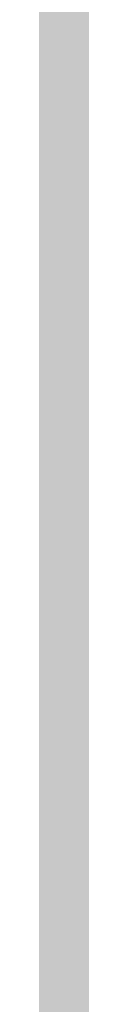
# Model space of a CAD drawing. Units: inches. Extents: x 2083 to 3317, y 1141 to 2115.
# Tile 180 of 256: x 3126.95594 to 3126.95825, y 1263.29018 to 1263.35483. Entities that reach past the tile are written whole.
import ezdxf

# ---------------------------------------------------------------- set-up
doc = ezdxf.new("R2010")
doc.units = ezdxf.units.IN
doc.layers.add('A-ANNO-DIMS', color=2, linetype='Continuous', lineweight=18)
doc.layers.add('A-WALL-PATT', color=251, linetype='Continuous', lineweight=13, true_color=0x636466)
doc.styles.get("Standard").update_dxf_attribs({"font": 'arial.ttf'})
doc.dimstyles.new('ISO-25', dxfattribs={"dimtxt": 12, "dimasz": 12, "dimexe": 1.25, "dimexo": 0.625, "dimtad": 1, "dimlunit": 3, "dimtxsty": 'Standard', "dimcen": 2.5, "dimadec": 0, "dimazin": 0, "dimtfac": 1, "dimtmove": 0, "dimatfit": 3, "dimfxl": 1, "dimarcsym": 0})

# ---------------------------------------------------------------- blocks, each defined once
blk = doc.blocks.new('*D26')
at = {"layer": 'A-ANNO-DIMS', "color": 0, "lineweight": -2, "transparency": 16777216}
for p, q in [((3088.985844, 1274.915092), (3088.985844, 1270.951963)), ((3111.240037, 1274.915092), (3111.240037, 1270.951963)), ((3076.985844, 1272.201963), (2840.262447, 1272.201963)), ((3111.240037, 1272.201963), (3088.985844, 1272.201963)), ((3123.240037, 1272.201963), (3135.240037, 1272.201963))]:
    blk.add_line(p, q, dxfattribs=at)
at = {"layer": 'A-ANNO-DIMS', "color": 0, "transparency": 16777216}
for points in [[(3076.985844, 1274.201963), (3076.985844, 1270.201963), (3088.985844, 1272.201963)], [(3123.240037, 1274.201963), (3123.240037, 1270.201963), (3111.240037, 1272.201963)]]:
    blk.add_solid(points, dxfattribs=at)
at = {"layer": 'Defpoints', "color": 0, "transparency": 16777216}
for p in [(3088.985844, 1275.540092), (3111.240037, 1275.540092), (3088.985844, 1272.201963)]:
    blk.add_point(p, dxfattribs=at)
at = {"layer": 'A-ANNO-DIMS', "color": 0, "transparency": 16777216, "insert": (2952.624146, 1279.031602), "char_height": 12, "attachment_point": 5}
blk.add_mtext('NIGHTSTAND 1\'-10 1/2" TYP.', dxfattribs=at)
blk = doc.blocks.new('*D27')
at = {"layer": 'A-ANNO-DIMS', "color": 0, "lineweight": -2, "transparency": 16777216}
for p, q in [((3114.578165, 1309.794285), (3114.578165, 1321.794285)), ((3111.865037, 1297.794285), (3115.828165, 1297.794285)), ((3114.578165, 1297.794285), (3114.578165, 1275.540092)), ((3111.865037, 1275.540092), (3115.828165, 1275.540092)), ((3114.578165, 1263.540092), (3114.578165, 1140.988591))]:
    blk.add_line(p, q, dxfattribs=at)
at = {"layer": 'A-ANNO-DIMS', "color": 0, "transparency": 16777216}
for points in [[(3112.578165, 1309.794285), (3116.578165, 1309.794285), (3114.578165, 1297.794285)], [(3112.578165, 1263.540092), (3116.578165, 1263.540092), (3114.578165, 1275.540092)]]:
    blk.add_solid(points, dxfattribs=at)
at = {"layer": 'Defpoints', "color": 0, "transparency": 16777216}
for p in [(3111.240037, 1297.794285), (3111.240037, 1275.540092), (3114.578165, 1275.540092)]:
    blk.add_point(p, dxfattribs=at)
at = {"layer": 'A-ANNO-DIMS', "color": 0, "transparency": 16777216, "insert": (3107.748527, 1196.264342), "char_height": 12, "attachment_point": 5, "rotation": 90}
blk.add_mtext('1\'-10 1/2" TYP.', dxfattribs=at)

msp = doc.modelspace()

# ---------------------------------------------------------------- hatches: boundary and pattern name
at = {"layer": 'A-WALL-PATT'}
h = msp.add_hatch(color=256, dxfattribs=at)
h.dxf.hatch_style = 1
h.paths.add_polyline_path([(3126.959783, 2020.76136), (2748.959783, 2020.76136), (2604.959783, 2020.76136), (2226.959783, 2020.76136), (2226.959783, 1702.76136), (2466.959783, 1702.76136), (2466.959783, 1582.76136), (2418.959783, 1582.76136), (2418.959783, 1477.76136), (2226.959783, 1477.76136), (2226.959783, 1263.26136), (2544.959783, 1263.26136), (2544.959783, 1411.76136), (2604.959783, 1411.76136), (2685.959783, 1411.76136), (2685.959783, 1420.76136), (2604.959783, 1420.76136), (2604.959783, 1573.76136), (2604.959783, 1702.76136), (2604.959783, 2011.76136), (2748.959783, 2011.76136), (2748.959783, 1702.76136), (2862.959783, 1702.76136), (2862.959783, 1621.76136), (2871.959783, 1621.76136), (2871.959783, 1702.76136), (2883.959783, 1702.76136), (2883.959783, 1706.939459, -0.026459), (2883.959783, 1711.76136), (2757.959783, 1711.76136), (2757.959783, 1807.76136), (2787.959783, 1807.76136), (2787.959783, 1812.26136), (2757.959783, 1812.26136), (2757.959783, 2011.76136), (2877.959783, 2011.76136), (2877.959783, 1812.26136), (2847.959783, 1812.26136), (2847.959783, 1807.76136), (2889.835742, 1807.76136), (2889.835742, 1812.26136), (2882.459783, 1812.26136), (2882.459783, 2011.76136), (3117.959783, 2011.76136), (3117.959783, 1812.26136), (2937.835742, 1812.26136), (2937.835742, 1807.76136), (2995.709783, 1807.76136), (2995.709783, 1796.117666), (3000.209783, 1796.117666), (3000.209783, 1807.76136), (3117.959783, 1807.76136), (3117.959783, 1711.76136), (3000.209783, 1711.76136), (3000.209783, 1760.117666), (2998.572705, 1760.117666, -0.020711), (2995.709783, 1760.117666), (2995.709783, 1711.76136), (2931.959783, 1711.76136), (2931.959783, 1702.76136), (3126.959783, 1702.76136)])
h.paths.add_polyline_path([(2471.459783, 2011.76136), (2471.459783, 1810.01136), (2462.716936, 1810.01136), (2462.716936, 1805.51136), (2505.959783, 1805.51136), (2505.959783, 1810.01136), (2475.959783, 1810.01136), (2475.959783, 2011.76136), (2595.959783, 2011.76136), (2595.959783, 1810.01136), (2565.959783, 1810.01136), (2565.959783, 1805.51136), (2595.959783, 1805.51136), (2595.959783, 1711.76136), (2235.959783, 1711.76136), (2235.959783, 1805.51136), (2353.709783, 1805.51136), (2353.709783, 1796.054162), (2358.209783, 1796.054162), (2358.209783, 1805.51136), (2414.716936, 1805.51136), (2414.716936, 1810.01136), (2235.959783, 1810.01136), (2235.959783, 2011.76136)], flags=16)
h.paths.add_polyline_path([(2270.204734, 1994.610008), (2270.204734, 1970.610008), (2246.204734, 1970.610008), (2246.204734, 1994.610008)], flags=0)
edge = h.paths.add_edge_path(flags=0)
edge.add_ellipse((2332.027391, 1899.798176), major_axis=(-3.042994, 3.042994), ratio=0.16825245, start_angle=-161.332166, end_angle=-156.307114, ccw=False)
edge.add_ellipse((2333.082037, 1898.74353), major_axis=(-1.054646, 1.054646), ratio=0.4535321, start_angle=-123.371019, end_angle=-94.159107)
edge = h.paths.add_edge_path(flags=0)
edge.add_ellipse((2332.027391, 1968.87629), major_axis=(3.042994, 3.042994), ratio=0.16825245, start_angle=18.667834, end_angle=23.692886)
edge.add_spline(control_points=[(2332.925596, 1970.691105), (2332.226768, 1970.3361), (2330.893709, 1969.658905), (2328.41308, 1970.932138), (2327.203934, 1967.748712), (2324.709596, 1969.955589), (2322.532822, 1967.012354), (2320.012846, 1971.295812), (2317.680308, 1968.157845), (2316.040526, 1967.102047), (2315.426904, 1966.809602)], knot_values=[0, 0, 0, 0, 2.267059, 4.324559, 6.685584, 8.878641, 11.121502, 14.300359, 17.755284, 19.732645, 19.732645, 19.732645, 19.732645], degree=3, periodic=0)
edge.add_ellipse((2332.027391, 1968.87629), major_axis=(3.042994, 3.042994), ratio=0.16825245, start_angle=18.667834, end_angle=23.692886, ccw=False)
edge.add_ellipse((2333.082037, 1969.930936), major_axis=(1.054646, 1.054646), ratio=0.4535321, start_angle=56.628981, end_angle=85.840893, ccw=False)
edge = h.paths.add_edge_path(flags=0)
edge.add_spline(control_points=[(2296.428287, 1967.987908), (2293.627804, 1965.336314), (2287.703624, 1959.727094), (2299.74386, 1949.995699), (2294.532591, 1935.668528), (2290.573228, 1920.603512), (2293.394124, 1909.973691), (2296.185407, 1904.966543)], knot_values=[0.099185, 0.099185, 0.099185, 0.099185, 0.345301, 0.619822, 0.982653, 1.386093, 1.810555, 1.810555, 1.810555, 1.810555], degree=3, periodic=0)
edge.add_spline(control_points=[(2296.185407, 1904.966543), (2297.383582, 1902.6193), (2298.000969, 1901.949312), (2298.55297, 1901.468155)], knot_values=[0.006246, 0.006246, 0.006246, 0.006246, 0.055476, 0.055476, 0.055476, 0.055476], degree=3, periodic=0)
edge.add_spline(control_points=[(2298.55297, 1901.468155), (2297.258612, 1900.923224), (2295.225294, 1900.232126), (2293.060229, 1900.614205), (2292.101423, 1900.788415), (2292.089578, 1900.790568)], knot_values=[0.312835, 0.312835, 0.312835, 0.312835, 0.40178, 0.474987, 0.475903, 0.475903, 0.475903, 0.475903], degree=3, periodic=0)
edge.add_arc((2292.793646, 1904.664109), 3.937008, 215.420897, 259.698179, ccw=False)
edge.add_spline(control_points=[(2289.585314, 1902.382304), (2289.476652, 1902.535087), (2289.36848, 1902.688035), (2289.260865, 1902.84117)], knot_values=[0.102872, 0.102872, 0.102872, 0.102872, 0.116896, 0.116896, 0.116896, 0.116896], degree=3, periodic=0)
edge.add_spline(control_points=[(2289.260865, 1902.84117), (2288.686604, 1902.550192), (2287.640048, 1902.019902), (2285.881337, 1901.873954), (2283.852972, 1901.504352), (2281.719987, 1899.710538), (2278.466991, 1899.492942), (2276.157136, 1901.883202), (2272.258953, 1899.804071), (2267.777605, 1901.843183), (2262.243882, 1900.184033), (2257.414927, 1901.782061), (2254.318374, 1900.72612), (2253.178285, 1900.337343)], knot_values=[0, 0, 0, 0, 1.907977, 3.477176, 5.261074, 7.972851, 11.680248, 13.717921, 16.939592, 22.789562, 27.502503, 33.595215, 37.145618, 37.145618, 37.145618, 37.145618], degree=3, periodic=0)
edge.add_line((2253.178285, 1900.337343), (2250.24424, 1902.84117))
edge.add_line((2250.24424, 1902.84117), (2250.24424, 1965.833296))
edge.add_line((2250.24424, 1965.833296), (2253.178285, 1968.337123))
edge.add_spline(control_points=[(2253.178285, 1968.337123), (2254.318374, 1967.948346), (2257.414927, 1966.892405), (2262.243882, 1968.490433), (2267.777605, 1966.831283), (2271.52673, 1968.537217), (2273.875914, 1967.828289), (2274.206701, 1967.727642)], knot_values=[0, 0, 0, 0, 0.09018, 0.244935, 0.364644, 0.513233, 0.537855, 0.537855, 0.537855, 0.537855], degree=3, periodic=0)
edge.add_arc((2274.352887, 1963.793349), 3.937008, 72.051134, 92.127949, ccw=False)
edge.add_arc((2281.296933, 1985.230003), 18.596298, 252.0511336, 288.5657217)
edge.add_arc((2292.316717, 1956.02888), 12.646081, 71.0267879, 113.7782184, ccw=False)
edge = h.paths.add_edge_path(flags=0)
edge.add_spline(control_points=[(2274.899415, 1951.856195), (2275.066156, 1951.616592), (2275.232687, 1951.376588), (2275.397987, 1951.135855)], knot_values=[1.409916, 1.409916, 1.409916, 1.409916, 1.43159, 1.43159, 1.43159, 1.43159], degree=3, periodic=0)
edge.add_spline(control_points=[(2275.397987, 1951.135855), (2275.792106, 1950.561885), (2276.179231, 1949.983774), (2276.545546, 1949.397103)], knot_values=[1.358238, 1.358238, 1.358238, 1.358238, 1.409916, 1.409916, 1.409916, 1.409916], degree=3, periodic=0)
edge.add_line((2276.545546, 1949.397103), (2277.437289, 1947.862185))
edge.add_spline(control_points=[(2277.437289, 1947.862185), (2276.303834, 1945.673115), (2274.639698, 1942.426882), (2274.631615, 1938.0939), (2272.799124, 1930.85155), (2274.356426, 1943.897046), (2275.947681, 1947.923356), (2276.545546, 1949.397103)], knot_values=[0.005632, 0.005632, 0.005632, 0.005632, 0.186014, 0.266002, 0.357087, 0.59639, 0.739732, 0.739732, 0.739732, 0.739732], degree=3, periodic=0)
edge.add_spline(control_points=[(2276.545546, 1949.397103), (2276.179231, 1949.983774), (2275.792106, 1950.561885), (2275.397987, 1951.135855)], knot_values=[1.358238, 1.358238, 1.358238, 1.358238, 1.409916, 1.409916, 1.409916, 1.409916], degree=3, periodic=0)
edge.add_spline(control_points=[(2275.397987, 1951.135855), (2274.9425, 1950.080452), (2274.20776, 1948.025272), (2273.934602, 1944.851477), (2272.468534, 1937.627489), (2273.466216, 1945.696466), (2274.700615, 1951.059472), (2274.899415, 1951.856195)], knot_values=[0.104364, 0.104364, 0.104364, 0.104364, 0.189636, 0.269624, 0.36071, 0.600013, 0.644622, 0.644622, 0.644622, 0.644622], degree=3, periodic=0)
h.paths.add_polyline_path([(2269.167514, 1963.127573, -0.357527), (2268.170633, 1960.97637, -0.092561), (2268.170633, 1939.436325, -0.357527), (2269.167514, 1937.285122, -0.357527), (2267.01631, 1938.282002, -0.164785), (2254.685581, 1938.282002, -0.357527), (2252.534378, 1937.285122, -0.357527), (2253.531259, 1939.436325, -0.092561), (2253.531259, 1960.97637, -0.357527), (2252.534378, 1963.127573, -0.357527), (2254.685581, 1962.130692, -0.164785), (2267.01631, 1962.130692, -0.357527)], flags=0)
h.paths.add_polyline_path([(2248.874068, 1967.8018), (2248.874068, 1957.02771), (2249.457783, 1957.02771), (2249.457783, 1911.646756), (2248.874068, 1911.646756), (2248.874068, 1900.872666), (2246.511863, 1900.872666, 0.197327), (2244.149658, 1902.456873), (2244.149658, 1966.217592, 0.197327), (2246.511863, 1967.8018)], flags=0)
h.paths.add_polyline_path([(2269.167514, 1931.389344, -0.357527), (2268.170633, 1929.238141, -0.092561), (2268.170633, 1907.698096, -0.357527), (2269.167514, 1905.546893, -0.357527), (2267.01631, 1906.543774, -0.164785), (2254.685581, 1906.543774, -0.357527), (2252.534378, 1905.546893, -0.357527), (2253.531259, 1907.698096, -0.092561), (2253.531259, 1929.238141, -0.357527), (2252.534378, 1931.389344, -0.357527), (2254.685581, 1930.392463, -0.164785), (2267.01631, 1930.392463, -0.357527)], flags=0)
edge = h.paths.add_edge_path(flags=0)
edge.add_spline(control_points=[(2276.196858, 1906.723702), (2276.168144, 1909.028928), (2276.114049, 1913.371852), (2270.598417, 1924.924978), (2273.905175, 1919.012779), (2275.921711, 1916.262063), (2275.47457, 1912.402149), (2277.257874, 1910.380621), (2276.696044, 1908.225036), (2276.646218, 1906.813023), (2276.617825, 1906.008407)], knot_values=[0, 0, 0, 0, 8.61026, 16.221274, 18.843057, 23.804898, 27.440828, 29.356102, 31.203478, 33.650687, 33.650687, 33.650687, 33.650687], degree=3, periodic=0)
edge.add_spline(control_points=[(2276.617825, 1906.008407), (2276.623313, 1905.624144), (2276.497738, 1904.628661), (2275.441779, 1903.854725), (2274.937314, 1903.08045), (2274.85908, 1902.84117)], knot_values=[0.156488, 0.156488, 0.156488, 0.156488, 0.184398, 0.231376, 0.250598, 0.250598, 0.250598, 0.250598], degree=3, periodic=0)
edge.add_line((2274.85908, 1902.84117), (2276.50598, 1902.84117))
edge.add_spline(control_points=[(2276.50598, 1902.84117), (2276.788308, 1903.08494), (2277.665071, 1904.125196), (2278.249538, 1904.340738), (2277.653872, 1908.527387), (2278.15567, 1906.227808), (2278.100464, 1905.285948), (2278.846675, 1904.069005), (2277.856785, 1903.414948), (2277.874191, 1902.99105), (2277.903562, 1902.84117)], knot_values=[0.059574, 0.059574, 0.059574, 0.059574, 0.080753, 0.103741, 0.16972, 0.176036, 0.207137, 0.240474, 0.262341, 0.27366, 0.27366, 0.27366, 0.27366], degree=3, periodic=0)
edge.add_line((2277.903562, 1902.84117), (2280.029825, 1902.84117))
edge.add_spline(control_points=[(2280.029825, 1902.84117), (2279.888221, 1903.088398), (2279.499257, 1903.981551), (2280.152284, 1905.939349), (2278.103615, 1909.657757), (2279.762395, 1907.185285), (2280.3279, 1904.874861), (2280.485109, 1903.48959), (2281.463269, 1903.249432), (2281.758343, 1902.936497), (2281.834036, 1902.84117)], knot_values=[0.013856, 0.013856, 0.013856, 0.013856, 0.034874, 0.088867, 0.107879, 0.126738, 0.158714, 0.193757, 0.217487, 0.226722, 0.226722, 0.226722, 0.226722], degree=3, periodic=0)
edge.add_spline(control_points=[(2281.834036, 1902.84117), (2281.787535, 1902.826703), (2281.647022, 1902.782988), (2281.395527, 1902.85949), (2281.088077, 1902.985242), (2280.720683, 1903.060902), (2280.333451, 1903.025726), (2280.124767, 1902.898879), (2280.029825, 1902.84117)], knot_values=[0, 0, 0, 0, 0.14413, 0.435517, 0.749276, 1.153046, 1.548371, 1.878348, 1.878348, 1.878348, 1.878348], degree=3, periodic=0)
edge.add_line((2280.029825, 1902.84117), (2277.903562, 1902.84117))
edge.add_spline(control_points=[(2277.903562, 1902.84117), (2277.892855, 1902.795855), (2277.865396, 1902.679637), (2277.607479, 1902.687483), (2277.27405, 1902.8007), (2276.837921, 1902.619775), (2276.583807, 1902.789261), (2276.50598, 1902.84117)], knot_values=[0, 0, 0, 0, 0.127189, 0.326199, 0.628009, 1.24357, 1.515331, 1.515331, 1.515331, 1.515331], degree=3, periodic=0)
edge.add_line((2276.50598, 1902.84117), (2274.85908, 1902.84117))
edge.add_spline(control_points=[(2274.85908, 1902.84117), (2274.814437, 1902.898587), (2274.72513, 1903.013446), (2274.493477, 1903.118968), (2274.244285, 1902.960539), (2273.937121, 1903.184942), (2273.614039, 1902.983143), (2273.408316, 1902.883045), (2273.322254, 1902.84117)], knot_values=[0, 0, 0, 0, 0.21843, 0.436957, 0.687977, 0.990379, 1.398396, 1.69185, 1.69185, 1.69185, 1.69185], degree=3, periodic=0)
edge.add_spline(control_points=[(2273.322254, 1902.84117), (2273.61674, 1903.445692), (2274.273998, 1904.538253), (2276.027239, 1904.573702), (2276.206963, 1906.583637), (2276.196858, 1906.723702)], knot_values=[0.012227, 0.012227, 0.012227, 0.012227, 0.059472, 0.106218, 0.134458, 0.134458, 0.134458, 0.134458], degree=3, periodic=0)
h.paths.add_polyline_path([(2270.776054, 1897.789828), (2270.776054, 1873.789828), (2246.776054, 1873.789828), (2246.776054, 1897.789828)], flags=0)
h.paths.add_polyline_path([(2353.709783, 1760.005059), (2353.709783, 1760.054162), (2358.209783, 1760.054162, -0.033729)], flags=0)
h.paths.add_polyline_path([(2321.819119, 1737.529186), (2341.995327, 1737.529186, -0.414214), (2343.203273, 1736.321241), (2343.203273, 1721.020596, -0.414214), (2341.995327, 1719.812651), (2321.819119, 1719.812651, -0.414214), (2320.611173, 1721.020596), (2320.611173, 1736.321241, -0.414214)], flags=0)
h.paths.add_polyline_path([(2324.23501, 1736.321241), (2339.579436, 1736.321241, -0.414214), (2341.995327, 1733.905349), (2341.995327, 1725.44973, -0.414214), (2339.579436, 1723.033839), (2333.680588, 1723.033839), (2333.845317, 1722.045467, -0.870646), (2335.425399, 1721.825893, -0.767327), (2333.922694, 1721.423245), (2331.291024, 1721.423245, -0.767327), (2329.788319, 1721.825893, -0.870646), (2331.368401, 1722.045467), (2331.53313, 1723.033839), (2324.23501, 1723.033839, -0.414214), (2321.819119, 1725.44973), (2321.819119, 1733.905349, -0.414214)], flags=0)
h.paths.add_polyline_path([(2570.483789, 1928.615444), (2589.683789, 1928.615444), (2590.168829, 1928.615444), (2590.168829, 1904.993397), (2570.483789, 1904.993397)], flags=0)
h.paths.add_polyline_path([(2574.447324, 1927.263822, -1), (2572.828836, 1927.263822, -1)], flags=0)
h.paths.add_polyline_path([(2573.089867, 1926.940877), (2573.925032, 1927.776042), (2574.147743, 1927.553332), (2573.312577, 1926.718166)], flags=0)
h.paths.add_polyline_path([(2578.779065, 1919.729618, -1), (2571.591663, 1919.729618, -1)], flags=0)
h.paths.add_polyline_path([(2578.385364, 1919.729618, -1), (2571.985364, 1919.729618, -1)], flags=0)
h.paths.add_polyline_path([(2331.595764, 1729.476216, -1), (2333.617954, 1729.476216, -1)], flags=0)
h.paths.add_polyline_path([(2578.034228, 1927.263822, -1), (2576.41574, 1927.263822, -1)], flags=0)
h.paths.add_polyline_path([(2576.688851, 1927.531089), (2576.911562, 1927.753799), (2577.746728, 1926.918634), (2577.524017, 1926.695923)], flags=0)
h.paths.add_polyline_path([(2578.139065, 1909.859539, -1), (2572.231663, 1909.859539, -1)], flags=0)
h.paths.add_polyline_path([(2577.745364, 1909.859539, -1), (2572.625364, 1909.859539, -1)], flags=0)
h.paths.add_polyline_path([(2583.797718, 1927.263822, -1), (2582.179229, 1927.263822, -1)], flags=0)
h.paths.add_polyline_path([(2582.718649, 1927.753799), (2583.553814, 1926.918634), (2583.331103, 1926.695923), (2582.495938, 1927.531089)], flags=0)
h.paths.add_polyline_path([(2582.495938, 1927.531089), (2582.718649, 1927.753799), (2583.553814, 1926.918634), (2583.331103, 1926.695923)], flags=0)
h.paths.add_polyline_path([(2587.739065, 1920.529618, -1), (2581.831663, 1920.529618, -1)], flags=0)
h.paths.add_polyline_path([(2587.345364, 1920.529618, -1), (2582.225364, 1920.529618, -1)], flags=0)
h.paths.add_polyline_path([(2587.384622, 1927.263822, -1), (2585.766133, 1927.263822, -1)], flags=0)
h.paths.add_polyline_path([(2586.081993, 1926.980247), (2586.917158, 1927.815412), (2587.139869, 1927.592702), (2586.304703, 1926.757536)], flags=0)
h.paths.add_polyline_path([(2588.379065, 1910.659539, -1), (2581.191663, 1910.659539, -1)], flags=0)
h.paths.add_polyline_path([(2587.985364, 1910.659539, -1), (2581.585364, 1910.659539, -1)], flags=0)
h.paths.add_polyline_path([(2417.167729, 1729.477895), (2437.343937, 1729.477895, -0.414214), (2438.551883, 1728.26995), (2438.551883, 1712.969306, -0.414214), (2437.343937, 1711.76136), (2417.167729, 1711.76136, -0.414214), (2415.959783, 1712.969306), (2415.959783, 1728.26995, -0.414214)], flags=0)
h.paths.add_polyline_path([(2419.58362, 1728.26995), (2434.928046, 1728.26995, -0.414214), (2437.343937, 1725.854059), (2437.343937, 1717.39844, -0.414214), (2434.928046, 1714.982548), (2429.029199, 1714.982548), (2429.193927, 1713.994176, -0.870646), (2430.774009, 1713.774603, -0.767327), (2429.271304, 1713.371954), (2426.639634, 1713.371954, -0.767327), (2425.136929, 1713.774603, -0.870646), (2426.717011, 1713.994176), (2426.88174, 1714.982548), (2419.58362, 1714.982548, -0.414214), (2417.167729, 1717.39844), (2417.167729, 1725.854059, -0.414214)], flags=0)
h.paths.add_polyline_path([(2419.58362, 1728.26995), (2434.928046, 1728.26995, -0.414214), (2437.343937, 1725.854059), (2437.343937, 1717.39844, -0.414214), (2434.928046, 1714.982548), (2429.029199, 1714.982548), (2428.358118, 1719.009034), (2427.552821, 1719.009034), (2426.88174, 1714.982548), (2419.58362, 1714.982548, -0.414214), (2417.167729, 1717.39844), (2417.167729, 1725.854059, -0.414214)], flags=0)
h.paths.add_polyline_path([(2426.944374, 1721.424925, -1), (2428.966564, 1721.424925, -1)], flags=0)
h.paths.add_polyline_path([(2475.959783, 1702.76136), (2595.959783, 1702.76136), (2595.959783, 1582.76136), (2475.959783, 1582.76136)], flags=16)
h.paths.add_polyline_path([(2427.959783, 1573.76136), (2595.959783, 1573.76136), (2595.959783, 1468.76136), (2595.959783, 1420.76136), (2384.459783, 1420.76136), (2384.459783, 1468.76136), (2427.959783, 1468.76136)], flags=16)
h.paths.add_polyline_path([(2379.959783, 1468.76136), (2379.959783, 1420.76136), (2235.959783, 1420.76136), (2235.959783, 1468.76136)], flags=16)
h.paths.add_polyline_path([(2317.815996, 1466.695767), (2337.992205, 1466.695767, -0.414214), (2339.20015, 1465.487821), (2339.20015, 1450.187177, -0.414214), (2337.992205, 1448.979232), (2317.815996, 1448.979232, -0.414214), (2316.608051, 1450.187177), (2316.608051, 1465.487821, -0.414214)], flags=0)
h.paths.add_polyline_path([(2320.231887, 1465.487821), (2335.576313, 1465.487821, -0.414214), (2337.992205, 1463.07193), (2337.992205, 1454.616311, -0.414214), (2335.576313, 1452.20042), (2329.677466, 1452.20042), (2329.842195, 1451.212047, -0.870646), (2331.422276, 1450.992474, -0.767327), (2329.919571, 1450.589826), (2327.287902, 1450.589826, -0.767327), (2325.785197, 1450.992474, -0.870646), (2327.365278, 1451.212047), (2327.530007, 1452.20042), (2320.231887, 1452.20042, -0.414214), (2317.815996, 1454.616311), (2317.815996, 1463.07193, -0.414214)], flags=0)
h.paths.add_polyline_path([(2320.231887, 1465.487821), (2335.576313, 1465.487821, -0.414214), (2337.992205, 1463.07193), (2337.992205, 1454.616311, -0.414214), (2335.576313, 1452.20042), (2329.677466, 1452.20042), (2329.006385, 1456.226905), (2328.201088, 1456.226905), (2327.530007, 1452.20042), (2320.231887, 1452.20042, -0.414214), (2317.815996, 1454.616311), (2317.815996, 1463.07193, -0.414214)], flags=0)
h.paths.add_polyline_path([(2327.592641, 1458.642796, -1), (2329.614832, 1458.642796, -1)], flags=0)
h.paths.add_polyline_path([(2244.411744, 1433.340453), (2241.920945, 1433.340453, -0.414214), (2240.017856, 1435.243542), (2240.017856, 1440.952808, -0.414211), (2241.920925, 1442.855897), (2244.411744, 1442.855897, -1.976472)], flags=0)
h.paths.add_polyline_path([(2245.356888, 1434.397536, -0.414214), (2245.356888, 1441.798814, -2.144098)], flags=0)
h.paths.add_polyline_path([(2535.959783, 1416.26136), (2535.959783, 1272.26136), (2235.959783, 1272.26136), (2235.959783, 1416.26136)], flags=16)
h.paths.add_polyline_path([(2260.119561, 1384.292841), (2260.119561, 1362.038649), (2237.865369, 1362.038649), (2237.865369, 1384.292841)], flags=0)
edge = h.paths.add_edge_path(flags=0)
edge.add_line((2318.251847, 1362.093298), (2318.145797, 1362.000973))
edge.add_ellipse((2317.445116, 1360.431044), major_axis=(2.82164, 2.82164), ratio=0.16825245, start_angle=18.667834, end_angle=20.948127, ccw=False)
edge.add_ellipse((2318.423045, 1361.408974), major_axis=(0.977929, 0.977929), ratio=0.4535321, start_angle=56.628981, end_angle=70.226201, ccw=False)
edge = h.paths.add_edge_path(flags=0)
edge.add_line((2319.10737, 1295.571078), (2319.015044, 1295.677128))
edge.add_ellipse((2317.445116, 1296.377809), major_axis=(-2.82164, 2.82164), ratio=0.16825245, start_angle=-161.332166, end_angle=-159.051873, ccw=False)
edge.add_ellipse((2318.423045, 1295.39988), major_axis=(-0.977929, 0.977929), ratio=0.4535321, start_angle=-123.371019, end_angle=-109.773799)
edge = h.paths.add_edge_path(flags=0)
edge.add_spline(control_points=[(2284.210349, 1301.170219), (2284.580688, 1300.444719), (2284.891189, 1299.892024), (2285.159553, 1299.461018)], knot_values=[0.039066, 0.039066, 0.039066, 0.039066, 0.055476, 0.055476, 0.055476, 0.055476], degree=3, periodic=0)
edge.add_line((2285.159553, 1299.461018), (2284.210349, 1301.170219))
edge = h.paths.add_edge_path(flags=0)
edge.add_line((2280.412458, 1297.298013), (2283.369991, 1297.036122))
edge.add_line((2283.369991, 1297.036122), (2286.40569, 1297.92631))
edge.add_spline(control_points=[(2286.40569, 1297.92631), (2285.305487, 1297.463119), (2284.344777, 1297.129151), (2283.369991, 1297.036122)], knot_values=[0.394369, 0.394369, 0.394369, 0.394369, 0.475903, 0.475903, 0.475903, 0.475903], degree=3, periodic=0)
edge.add_spline(control_points=[(2283.369991, 1297.036122), (2283.28139, 1297.027666), (2282.316289, 1296.957336), (2281.312502, 1297.134479), (2280.423441, 1297.296016), (2280.412458, 1297.298013)], knot_values=[0.312835, 0.312835, 0.312835, 0.312835, 0.320246, 0.393453, 0.394369, 0.394369, 0.394369, 0.394369], degree=3, periodic=0)
edge = h.paths.add_edge_path(flags=0)
edge.add_line((2284.435561, 1359.607285), (2280.446291, 1355.328047))
edge.add_line((2280.446291, 1355.328047), (2279.579987, 1351.017754))
edge.add_line((2279.579987, 1351.017754), (2282.412974, 1346.580433))
edge.add_spline(control_points=[(2282.412974, 1346.580433), (2283.153331, 1345.589236), (2284.252896, 1344.028897), (2284.801037, 1342.387167), (2284.935162, 1341.805544)], knot_values=[1.240098, 1.240098, 1.240098, 1.240098, 1.332892, 1.382712, 1.382712, 1.382712, 1.382712], degree=3, periodic=0)
edge.add_spline(control_points=[(2284.935162, 1341.805544), (2285.319108, 1340.1406), (2285.233029, 1338.409204), (2284.909938, 1336.654122)], knot_values=[1.097484, 1.097484, 1.097484, 1.097484, 1.240098, 1.240098, 1.240098, 1.240098], degree=3, periodic=0)
edge.add_spline(control_points=[(2284.909938, 1336.654122), (2284.586848, 1334.89904), (2284.026745, 1333.120272), (2283.462644, 1331.360585)], knot_values=[0.95487, 0.95487, 0.95487, 0.95487, 1.097484, 1.097484, 1.097484, 1.097484], degree=3, periodic=0)
edge.add_line((2283.462644, 1331.360585), (2281.890376, 1326.153357))
edge.add_line((2281.890376, 1326.153357), (2280.756259, 1321.056089))
edge.add_line((2280.756259, 1321.056089), (2280.299205, 1316.001977))
edge.add_line((2280.299205, 1316.001977), (2280.715933, 1310.950068))
edge.add_line((2280.715933, 1310.950068), (2282.028094, 1305.972137))
edge.add_line((2282.028094, 1305.972137), (2284.210349, 1301.170219))
edge.add_spline(control_points=[(2284.210349, 1301.170219), (2283.340731, 1302.730185), (2282.611904, 1304.336493), (2282.028094, 1305.972137)], knot_values=[0.099185, 0.099185, 0.099185, 0.099185, 0.241799, 0.241799, 0.241799, 0.241799], degree=3, periodic=0)
edge.add_spline(control_points=[(2282.028094, 1305.972137), (2281.444283, 1307.60778), (2281.005489, 1309.272759), (2280.715933, 1310.950068)], knot_values=[0.241799, 0.241799, 0.241799, 0.241799, 0.384413, 0.384413, 0.384413, 0.384413], degree=3, periodic=0)
edge.add_spline(control_points=[(2280.715933, 1310.950068), (2280.433241, 1312.587613), (2280.289386, 1314.276959), (2280.298894, 1315.962032), (2280.299205, 1316.001977)], knot_values=[0.384413, 0.384413, 0.384413, 0.384413, 0.523647, 0.527028, 0.527028, 0.527028, 0.527028], degree=3, periodic=0)
edge.add_spline(control_points=[(2280.299205, 1316.001977), (2280.312326, 1317.686955), (2280.477871, 1319.367926), (2280.756259, 1321.056089)], knot_values=[0.527028, 0.527028, 0.527028, 0.527028, 0.669642, 0.669642, 0.669642, 0.669642], degree=3, periodic=0)
edge.add_spline(control_points=[(2280.756259, 1321.056089), (2281.034648, 1322.744252), (2281.42588, 1324.439608), (2281.890376, 1326.153357)], knot_values=[0.669642, 0.669642, 0.669642, 0.669642, 0.812256, 0.812256, 0.812256, 0.812256], degree=3, periodic=0)
edge.add_spline(control_points=[(2281.890376, 1326.153357), (2282.264383, 1327.533251), (2282.78787, 1329.26181), (2283.352751, 1331.01778), (2283.462644, 1331.360585)], knot_values=[0.812256, 0.812256, 0.812256, 0.812256, 0.927087, 0.95487, 0.95487, 0.95487, 0.95487], degree=3, periodic=0)
edge.add_line((2283.462644, 1331.360585), (2284.909938, 1336.654122))
edge.add_line((2284.909938, 1336.654122), (2284.935162, 1341.805544))
edge.add_line((2284.935162, 1341.805544), (2282.412974, 1346.580433))
edge.add_spline(control_points=[(2282.412974, 1346.580433), (2281.275127, 1348.103792), (2280.078447, 1349.570318), (2279.579987, 1351.017754)], knot_values=[1.382712, 1.382712, 1.382712, 1.382712, 1.525326, 1.525326, 1.525326, 1.525326], degree=3, periodic=0)
edge.add_spline(control_points=[(2279.579987, 1351.017754), (2279.443282, 1351.414721), (2279.136312, 1352.856922), (2279.73519, 1354.290385), (2280.446291, 1355.328047)], knot_values=[1.525326, 1.525326, 1.525326, 1.525326, 1.564439, 1.667941, 1.667941, 1.667941, 1.667941], degree=3, periodic=0)
edge.add_spline(control_points=[(2280.446291, 1355.328047), (2281.426113, 1356.757835), (2282.930837, 1358.18256), (2284.435561, 1359.607285)], knot_values=[1.667941, 1.667941, 1.667941, 1.667941, 1.810555, 1.810555, 1.810555, 1.810555], degree=3, periodic=0)
edge.add_arc((2280.623075, 1348.518181), 11.72618, 71.0267879, 113.7782184)
edge.add_arc((2270.404892, 1375.595156), 17.243567, 252.0511336, 288.5657217, ccw=False)
edge.add_arc((2263.965969, 1355.717847), 3.650622, 72.051134, 92.127949)
edge.add_arc((2263.965969, 1355.717847), 3.650622, 92.127949, 177.98513)
edge.add_spline(control_points=[(2260.317604, 1355.846199), (2260.260417, 1354.220668), (2260.551278, 1350.186547), (2262.999344, 1346.766251), (2264.472741, 1344.649024)], knot_values=[1.43159, 1.43159, 1.43159, 1.43159, 1.564144, 1.770695, 1.770695, 1.770695, 1.770695], degree=3, periodic=0)
edge.add_line((2264.472741, 1344.649024), (2264.93559, 1343.98253))
edge.add_spline(control_points=[(2263.801044, 1340.248105), (2263.843238, 1340.514088), (2264.067244, 1341.756465), (2264.512693, 1343.002453), (2264.935047, 1343.981083)], knot_values=[0.53657, 0.53657, 0.53657, 0.53657, 0.559349, 0.644622, 0.644622, 0.644622, 0.644622], degree=3, periodic=0)
edge.add_spline(control_points=[(2264.935047, 1343.981083), (2265.117771, 1343.714975), (2265.298875, 1343.447906), (2265.476756, 1343.179365)], knot_values=[1.384077, 1.384077, 1.384077, 1.384077, 1.409916, 1.409916, 1.409916, 1.409916], degree=3, periodic=0)
edge.add_spline(control_points=[(2265.476756, 1343.179365), (2265.654637, 1342.910823), (2265.829296, 1342.64081), (2265.99913, 1342.368812)], knot_values=[1.358238, 1.358238, 1.358238, 1.358238, 1.384077, 1.384077, 1.384077, 1.384077], degree=3, periodic=0)
edge.add_line((2265.99913, 1342.368812), (2266.826006, 1340.945547))
edge.add_spline(control_points=[(2266.826006, 1340.945547), (2268.894401, 1337.089691), (2271.398173, 1325.843001), (2270.516164, 1310.568557), (2275.919376, 1301.860609), (2277.789511, 1299.19945)], knot_values=[0.116896, 0.116896, 0.116896, 0.116896, 0.472987, 1.050969, 1.313793, 1.313793, 1.313793, 1.313793], degree=3, periodic=0)
edge.add_spline(control_points=[(2277.789511, 1299.19945), (2277.839405, 1299.128452), (2277.889428, 1299.057498), (2277.939572, 1298.986584)], knot_values=[0.109884, 0.109884, 0.109884, 0.109884, 0.116896, 0.116896, 0.116896, 0.116896], degree=3, periodic=0)
edge.add_line((2277.939572, 1298.986584), (2277.788849, 1299.199114))
edge.add_spline(control_points=[(2277.788849, 1299.199114), (2277.256582, 1298.929414), (2276.28635, 1298.437902), (2275.039352, 1298.334419), (2274.38333, 1298.238895), (2274.215254, 1298.209338)], knot_values=[33.12187, 33.12187, 33.12187, 33.12187, 35.029056, 36.598255, 37.144827, 37.144827, 37.144827, 37.144827], degree=3, periodic=0)
edge.add_line((2274.215254, 1298.209338), (2273.073147, 1297.892961))
edge.add_spline(control_points=[(2273.073147, 1297.892961), (2272.322936, 1297.579784), (2271.039151, 1296.510508), (2269.248395, 1296.226062), (2268.4231, 1296.374654)], knot_values=[26.532584, 26.532584, 26.532584, 26.532584, 29.198919, 31.839101, 31.839101, 31.839101, 31.839101], degree=3, periodic=0)
edge.add_line((2268.4231, 1296.374654), (2263.878501, 1297.457534))
edge.add_spline(control_points=[(2263.878501, 1297.457534), (2263.556077, 1297.359435), (2261.860306, 1296.838694), (2260.23878, 1297.282407), (2258.933454, 1297.516461)], knot_values=[15.919551, 15.919551, 15.919551, 15.919551, 16.939592, 21.226067, 21.226067, 21.226067, 21.226067], degree=3, periodic=0)
edge.add_line((2258.933454, 1297.516461), (2254.055233, 1297.32901))
edge.add_spline(control_points=[(2254.055233, 1297.32901), (2253.755525, 1297.295815), (2252.113683, 1297.165174), (2250.461869, 1297.544221), (2249.129686, 1297.667882)], knot_values=[5.306517, 5.306517, 5.306517, 5.306517, 6.276435, 10.613034, 10.613034, 10.613034, 10.613034], degree=3, periodic=0)
edge.add_line((2249.129686, 1297.667882), (2244.33165, 1296.877756))
edge.add_line((2244.33165, 1296.877756), (2241.611033, 1299.19945))
edge.add_line((2241.611033, 1299.19945), (2241.611033, 1357.609404))
edge.add_line((2241.611033, 1357.609404), (2244.33165, 1359.931097))
edge.add_line((2244.33165, 1359.931097), (2252.728823, 1359.542692))
edge.add_spline(control_points=[(2252.728823, 1359.542692), (2252.870939, 1359.54644), (2253.30574, 1359.548172), (2253.739845, 1359.514274), (2254.031742, 1359.482426)], knot_values=[0.233291, 0.233291, 0.233291, 0.233291, 0.244935, 0.268927, 0.268927, 0.268927, 0.268927], degree=3, periodic=0)
edge.add_line((2254.031742, 1359.482426), (2259.58719, 1359.41639))
edge.add_spline(control_points=[(2259.58719, 1359.41639), (2260.677068, 1359.628503), (2262.073197, 1359.897003), (2263.523692, 1359.459278), (2263.830417, 1359.365952)], knot_values=[0.422516, 0.422516, 0.422516, 0.422516, 0.513233, 0.537855, 0.537855, 0.537855, 0.537855], degree=3, periodic=0)
edge.add_arc((2263.965969, 1355.717847), 3.650622, 72.051134, 92.127949, ccw=False)
edge.add_arc((2270.404892, 1375.595156), 17.243567, 252.0511336, 288.5657217)
edge.add_arc((2280.623075, 1348.518181), 11.72618, 71.0267879, 113.7782184, ccw=False)
h.paths.add_polyline_path([(2240.34053, 1359.434715), (2240.34053, 1349.444353), (2240.881785, 1349.444353), (2240.881785, 1307.3645), (2240.34053, 1307.3645), (2240.34053, 1297.374138), (2238.150157, 1297.374138, 0.197327), (2235.959783, 1298.843108), (2235.959783, 1357.965746, 0.197327), (2238.150157, 1359.434715)], flags=0)
h.paths.add_polyline_path([(2259.15779, 1355.1005, -0.357527), (2258.233425, 1353.10578, -0.092561), (2258.233425, 1333.132601, -0.357527), (2259.15779, 1331.13788, -0.357527), (2257.16307, 1332.062246, -0.164785), (2245.729302, 1332.062246, -0.357527), (2243.734582, 1331.13788, -0.357527), (2244.658947, 1333.132601, -0.092561), (2244.658947, 1353.10578, -0.357527), (2243.734582, 1355.1005, -0.357527), (2245.729302, 1354.176135, -0.164785), (2257.16307, 1354.176135, -0.357527)], flags=0)
edge = h.paths.add_edge_path(flags=0)
edge.add_line((2265.99913, 1342.368812), (2266.826006, 1340.945547))
edge.add_line((2266.826006, 1340.945547), (2265.307557, 1337.814066))
edge.add_line((2265.307557, 1337.814066), (2264.358232, 1334.652939))
edge.add_line((2264.358232, 1334.652939), (2264.262012, 1333.799705))
edge.add_spline(control_points=[(2264.262012, 1333.799705), (2264.208357, 1333.187055), (2264.16206, 1332.365525), (2264.007144, 1331.413933), (2263.969049, 1331.201834)], knot_values=[0.464444, 0.464444, 0.464444, 0.464444, 0.516691, 0.531608, 0.531608, 0.531608, 0.531608], degree=3, periodic=0)
edge.add_spline(control_points=[(2263.969049, 1331.201834), (2263.774535, 1330.118873), (2263.42437, 1328.790839), (2263.25742, 1328.530652), (2263.234028, 1328.514612)], knot_values=[0.372682, 0.372682, 0.372682, 0.372682, 0.44885, 0.464444, 0.464444, 0.464444, 0.464444], degree=3, periodic=0)
edge.add_spline(control_points=[(2263.234028, 1328.514612), (2263.096382, 1328.420227), (2263.13117, 1329.301477), (2263.274953, 1330.615749)], knot_values=[0.280919, 0.280919, 0.280919, 0.280919, 0.372682, 0.372682, 0.372682, 0.372682], degree=3, periodic=0)
edge.add_spline(control_points=[(2263.274953, 1330.615749), (2263.418736, 1331.930022), (2263.671515, 1333.677318), (2263.969852, 1335.315027)], knot_values=[0.189157, 0.189157, 0.189157, 0.189157, 0.280919, 0.280919, 0.280919, 0.280919], degree=3, periodic=0)
edge.add_spline(control_points=[(2263.969852, 1335.315027), (2264.100496, 1336.032192), (2264.418783, 1337.621911), (2264.754848, 1338.86443), (2264.947419, 1339.491124)], knot_values=[0.097394, 0.097394, 0.097394, 0.097394, 0.137578, 0.189157, 0.189157, 0.189157, 0.189157], degree=3, periodic=0)
edge.add_spline(control_points=[(2264.947419, 1339.491124), (2265.290017, 1340.606055), (2265.644238, 1341.493996), (2265.99913, 1342.368812)], knot_values=[0.005632, 0.005632, 0.005632, 0.005632, 0.097394, 0.097394, 0.097394, 0.097394], degree=3, periodic=0)
h.paths.add_polyline_path([(2259.15779, 1325.670973, -0.357527), (2258.233425, 1323.676253, -0.092561), (2258.233425, 1303.703073, -0.357527), (2259.15779, 1301.708353, -0.357527), (2257.16307, 1302.632719, -0.164785), (2245.729302, 1302.632719, -0.357527), (2243.734582, 1301.708353, -0.357527), (2244.658947, 1303.703073, -0.092561), (2244.658947, 1323.676253, -0.357527), (2243.734582, 1325.670973, -0.357527), (2245.729302, 1324.746608, -0.164785), (2257.16307, 1324.746608, -0.357527)], flags=0)
edge = h.paths.add_edge_path(flags=0)
edge.add_spline(control_points=[(2261.708938, 1317.311421), (2261.679482, 1317.41758), (2261.761858, 1317.388535), (2262.490736, 1316.089873), (2262.962185, 1315.300897)], knot_values=[14.955861, 14.955861, 14.955861, 14.955861, 16.221274, 18.694826, 18.694826, 18.694826, 18.694826], degree=3, periodic=0)
edge.add_spline(control_points=[(2262.962185, 1315.300897), (2262.990437, 1315.253617), (2263.702096, 1314.067376), (2264.348983, 1313.127153), (2264.730054, 1312.164154)], knot_values=[18.694826, 18.694826, 18.694826, 18.694826, 18.843057, 22.433791, 22.433791, 22.433791, 22.433791], degree=3, periodic=0)
edge.add_spline(control_points=[(2264.730054, 1312.164154), (2264.875565, 1311.796437), (2265.176873, 1310.769807), (2265.143069, 1309.559262), (2265.247736, 1308.824193)], knot_values=[22.433791, 22.433791, 22.433791, 22.433791, 23.804898, 26.172756, 26.172756, 26.172756, 26.172756], degree=3, periodic=0)
edge.add_line((2265.247736, 1308.824193), (2265.850774, 1307.171888))
edge.add_spline(control_points=[(2265.850774, 1307.171888), (2266.065025, 1306.821678), (2266.384387, 1306.332246), (2266.4244, 1305.780549), (2266.420369, 1305.611216)], knot_values=[28.062562, 28.062562, 28.062562, 28.062562, 29.356102, 29.911721, 29.911721, 29.911721, 29.911721], degree=3, periodic=0)
edge.add_spline(control_points=[(2266.420369, 1305.611216), (2266.416116, 1305.43259), (2266.393999, 1305.249998), (2266.364777, 1305.065857)], knot_values=[29.911721, 29.911721, 29.911721, 29.911721, 30.497837, 30.497837, 30.497837, 30.497837], degree=3, periodic=0)
edge.add_line((2266.364777, 1305.065857), (2266.066151, 1302.136295))
edge.add_spline(control_points=[(2266.066151, 1302.136295), (2266.07124, 1301.779984), (2265.998076, 1301.199985), (2265.663266, 1300.758961), (2265.508908, 1300.585882)], knot_values=[0.156488, 0.156488, 0.156488, 0.156488, 0.184398, 0.203543, 0.203543, 0.203543, 0.203543], degree=3, periodic=0)
edge.add_line((2265.508908, 1300.585882), (2264.435341, 1299.19945))
edge.add_line((2264.435341, 1299.19945), (2265.962442, 1299.19945))
edge.add_line((2265.962442, 1299.19945), (2267.33599, 1301.175276))
edge.add_line((2267.33599, 1301.175276), (2267.311667, 1301.986237))
edge.add_spline(control_points=[(2267.311667, 1301.986237), (2267.261111, 1302.862396), (2267.160212, 1303.737132), (2267.271486, 1303.325896)], knot_values=[0.126229, 0.126229, 0.126229, 0.126229, 0.166617, 0.166617, 0.166617, 0.166617], degree=3, periodic=0)
edge.add_spline(control_points=[(2267.271486, 1303.325896), (2267.280035, 1303.294305), (2267.309785, 1303.175366), (2267.37345, 1302.883608), (2267.406123, 1302.682829), (2267.417926, 1302.601025)], knot_values=[0.166617, 0.166617, 0.166617, 0.166617, 0.16972, 0.176036, 0.180765, 0.180765, 0.180765, 0.180765], degree=3, periodic=0)
edge.add_spline(control_points=[(2267.743891, 1300.987505), (2267.687583, 1301.150943), (2267.48052, 1301.656664), (2267.483751, 1302.144788), (2267.417926, 1302.601025)], knot_values=[0.180765, 0.180765, 0.180765, 0.180765, 0.193767, 0.220139, 0.220139, 0.220139, 0.220139], degree=3, periodic=0)
edge.add_line((2267.417926, 1302.601025), (2267.743891, 1300.987505))
edge.add_spline(control_points=[(2267.743891, 1300.987505), (2267.831961, 1300.731878), (2267.932021, 1300.309904), (2267.554841, 1299.974518), (2267.429366, 1299.829207)], knot_values=[0.220139, 0.220139, 0.220139, 0.220139, 0.240474, 0.25489, 0.25489, 0.25489, 0.25489], degree=3, periodic=0)
edge.add_line((2267.429366, 1299.829207), (2267.258361, 1299.19945))
edge.add_line((2267.258361, 1299.19945), (2269.229956, 1299.19945))
edge.add_spline(control_points=[(2269.229956, 1299.19945), (2269.098653, 1299.428694), (2268.842774, 1300.016251), (2269.011575, 1300.915923), (2268.946796, 1301.66074)], knot_values=[0.013856, 0.013856, 0.013856, 0.013856, 0.034874, 0.067073, 0.067073, 0.067073, 0.067073], degree=3, periodic=0)
edge.add_line((2268.946796, 1301.66074), (2268.431582, 1303.603109))
edge.add_spline(control_points=[(2268.431582, 1303.603109), (2268.175596, 1304.192375), (2267.596214, 1305.251298), (2268.040698, 1304.62321), (2268.251394, 1304.282421)], knot_values=[0.090155, 0.090155, 0.090155, 0.090155, 0.107879, 0.120289, 0.120289, 0.120289, 0.120289], degree=3, periodic=0)
edge.add_spline(control_points=[(2268.251394, 1304.282421), (2268.360882, 1304.105329), (2269.057753, 1302.917983), (2269.382691, 1301.590419), (2269.521405, 1300.775931), (2269.57522, 1300.555784)], knot_values=[0.120289, 0.120289, 0.120289, 0.120289, 0.126738, 0.158714, 0.173506, 0.173506, 0.173506, 0.173506], degree=3, periodic=0)
edge.add_line((2269.57522, 1300.555784), (2270.685798, 1299.421258))
edge.add_spline(control_points=[(2270.685798, 1299.421258), (2270.767221, 1299.357251), (2270.837852, 1299.281401), (2270.902925, 1299.19945)], knot_values=[0.21816, 0.21816, 0.21816, 0.21816, 0.226722, 0.226722, 0.226722, 0.226722], degree=3, periodic=0)
edge.add_line((2270.937201, 1299.192913), (2270.902925, 1299.19945))
edge.add_spline(control_points=[(2270.902925, 1299.19945), (2270.859806, 1299.186035), (2270.729515, 1299.1455), (2270.496314, 1299.216437), (2270.271661, 1299.308323), (2270.121017, 1299.347961), (2270.063339, 1299.359557)], knot_values=[0.939174, 0.939174, 0.939174, 0.939174, 1.083304, 1.374691, 1.68845, 1.878348, 1.878348, 1.878348, 1.878348], degree=3, periodic=0)
edge.add_line((2270.063339, 1299.359557), (2269.229956, 1299.19945))
edge.add_line((2269.229956, 1299.19945), (2267.258361, 1299.19945))
edge.add_spline(control_points=[(2267.258361, 1299.19945), (2267.248433, 1299.157431), (2267.222971, 1299.049667), (2266.983816, 1299.056942), (2266.80921, 1299.11623), (2266.676905, 1299.109091), (2266.636531, 1299.104815)], knot_values=[0.757665, 0.757665, 0.757665, 0.757665, 0.884854, 1.083864, 1.385675, 1.515331, 1.515331, 1.515331, 1.515331], degree=3, periodic=0)
edge.add_spline(control_points=[(2266.636531, 1299.104815), (2266.485225, 1299.088788), (2266.235807, 1299.017123), (2266.034608, 1299.151317), (2265.962442, 1299.19945)], knot_values=[0, 0, 0, 0, 0.485905, 0.757665, 0.757665, 0.757665, 0.757665], degree=3, periodic=0)
edge.add_line((2265.962442, 1299.19945), (2264.435341, 1299.19945))
edge.add_line((2264.435341, 1299.19945), (2263.858444, 1299.367118))
edge.add_spline(control_points=[(2263.858444, 1299.367118), (2263.818943, 1299.370905), (2263.779528, 1299.385721), (2263.740131, 1299.401504)], knot_values=[0.845925, 0.845925, 0.845925, 0.845925, 0.978627, 0.978627, 0.978627, 0.978627], degree=3, periodic=0)
edge.add_line((2263.721786, 1299.396425), (2263.010306, 1299.19945))
edge.add_spline(control_points=[(2263.010306, 1299.19945), (2263.245794, 1299.682859), (2263.506032, 1300.128107), (2263.873494, 1300.408028)], knot_values=[0.012227, 0.012227, 0.012227, 0.012227, 0.052971, 0.052971, 0.052971, 0.052971], degree=3, periodic=0)
edge.add_spline(control_points=[(2263.873494, 1300.408028), (2263.932131, 1300.452695), (2264.084243, 1300.552979), (2264.255189, 1300.624223), (2264.359686, 1300.664747)], knot_values=[0.052971, 0.052971, 0.052971, 0.052971, 0.059472, 0.069086, 0.069086, 0.069086, 0.069086], degree=3, periodic=0)
edge.add_line((2264.359686, 1300.664747), (2265.1419, 1301.077774))
edge.add_line((2265.1419, 1301.077774), (2265.675806, 1302.799558))
edge.add_line((2265.675806, 1302.799558), (2265.5407, 1305.704066))
edge.add_line((2265.5407, 1305.704066), (2264.803073, 1309.327724))
edge.add_line((2264.803073, 1309.327724), (2263.040535, 1314.091791))
edge.add_spline(control_points=[(2263.040535, 1314.091791), (2262.383572, 1315.671438), (2261.795972, 1316.997749), (2261.708938, 1317.311421)], knot_values=[11.216896, 11.216896, 11.216896, 11.216896, 14.955861, 14.955861, 14.955861, 14.955861], degree=3, periodic=0)
h.paths.add_polyline_path([(2871.959783, 1416.26136), (2895.910047, 1416.26136), (2895.910047, 1420.76136), (2871.959783, 1420.76136), (2871.959783, 1501.76136), (2862.959783, 1501.76136), (2862.959783, 1420.76136), (2805.959783, 1420.76136), (2805.959783, 1411.76136), (2862.959783, 1411.76136), (2862.959783, 1263.26136), (3126.959783, 1263.26136), (3126.959783, 1411.76136), (3126.959783, 1486.76136), (2943.959783, 1486.76136), (2943.959783, 1477.76136), (2967.860311, 1477.76136), (2967.860311, 1420.76136), (2943.910047, 1420.76136), (2943.910047, 1416.26136), (3117.959783, 1416.26136), (3117.959783, 1420.76136), (2972.360311, 1420.76136), (2972.360311, 1477.76136), (3117.959783, 1477.76136), (3117.959783, 1420.76136), (3117.959783, 1272.26136), (2871.959783, 1272.26136)], flags=0)
h.paths.add_polyline_path([(2457.125626, 1485.942505), (2527.602651, 1485.942505), (2527.602651, 1537.635702), (2457.125626, 1537.635702)], flags=8)
h.paths.add_polyline_path([(2481.005058, 1609.981804), (2590.765818, 1609.981804), (2590.765818, 1682.003362), (2481.005058, 1682.003362)], flags=8)
h.paths.add_polyline_path([(2483.085022, 1729.126784), (2553.562048, 1729.126784), (2553.562048, 1780.81998), (2483.085022, 1780.81998)], flags=8)
h = msp.add_hatch(color=256, dxfattribs=at)
h.dxf.hatch_style = 1
h.paths.add_polyline_path([(3126.959783, 1486.76136), (2943.959783, 1486.76136), (2943.959783, 1477.76136), (2967.860311, 1477.76136), (2967.860311, 1420.76136), (2943.910047, 1420.76136), (2943.910047, 1416.26136), (3117.959783, 1416.26136), (3117.959783, 1420.76136), (2972.360311, 1420.76136), (2972.360311, 1477.76136), (3117.959783, 1477.76136), (3117.959783, 1420.76136), (3117.959783, 1272.26136), (2871.959783, 1272.26136), (2871.959783, 1416.26136), (2895.910047, 1416.26136), (2895.910047, 1420.76136), (2871.959783, 1420.76136), (2871.959783, 1501.76136), (2862.959783, 1501.76136), (2862.959783, 1420.76136), (2805.959783, 1420.76136), (2805.959783, 1411.76136), (2862.959783, 1411.76136), (2862.959783, 1263.26136), (3126.959783, 1263.26136), (3126.959783, 1411.76136)])

# ---------------------------------------------------------------- dimensions: what is measured, and where the dimension line sits
at = {"layer": 'A-ANNO-DIMS'}
for base, p1, p2, angle, text, picture, middle in [((3114.578165, 1275.540092), (3111.240037, 1297.794285), (3111.240037, 1275.540092), 270, '<> TYP.', '*D27', (3107.748527, 1196.264342)), ((3088.985844, 1272.201963), (3111.240037, 1275.540092), (3088.985844, 1275.540092), 180, 'NIGHTSTAND <> TYP.', '*D26', (2952.624146, 1279.031602))]:
    dim = msp.add_linear_dim(base=base, p1=p1, p2=p2, angle=angle, text=text, dimstyle='ISO-25', override={"dimdec": 1, "dimlfac": 1, "dimrnd": 0, "dimzin": 1, "dimdsep": 46, "dimlunit": 4, "dimfrac": 2}, dxfattribs=at)
    dim.commit()
    dim.dimension.update_dxf_attribs({"geometry": picture, "text_midpoint": middle})

doc.saveas('drawing.dxf')
